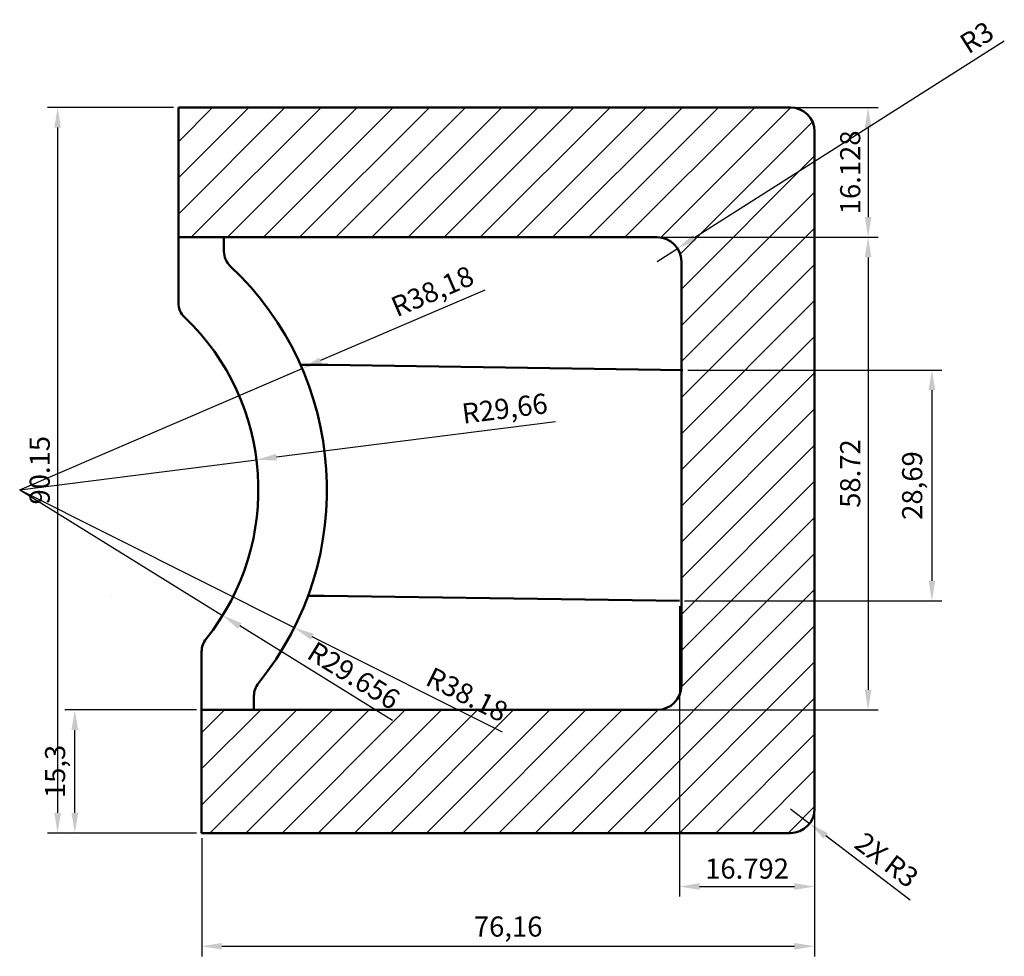
# Model space of a CAD drawing. Units: millimetres. Extents: x 1381 to 2009, y 1325 to 1613.
# Tile 6 of 6: x 1887 to 2009, y 1352 to 1468. Entities that reach past the tile are written whole.
import ezdxf

# ---------------------------------------------------------------- set-up
doc = ezdxf.new("R2010")
doc.units = ezdxf.units.MM
for name, color, linetype, lineweight in [('M-DIMS', 2, 'Continuous', 25), ('M-HATC', 8, 'Continuous', 18), ('M-OUTL', 7, 'Continuous', 50)]:
    doc.layers.add(name, color=color, linetype=linetype, lineweight=lineweight)
doc.styles.get("Standard").update_dxf_attribs({"font": 'arial.ttf'})
doc.dimstyles.new('ISO-25', dxfattribs={"dimtxt": 2.5, "dimasz": 2.5, "dimexe": 1.25, "dimexo": 0.625, "dimtad": 1, "dimtxsty": 'Standard', "dimcen": 2.5, "dimadec": 0, "dimazin": 0, "dimtfac": 1, "dimtmove": 0, "dimatfit": 3, "dimfxl": 1, "dimarcsym": 0})

# ---------------------------------------------------------------- blocks, each defined once
blk = doc.blocks.new('*D32')
at = {"layer": 'Defpoints', "color": 0, "transparency": 16777216}
for p in [(1968.55, 1439.75), (1966.02, 1438.15)]:
    blk.add_point(p, dxfattribs=at)
at = {"layer": 'M-DIMS', "color": 0, "lineweight": -2, "transparency": 16777216}
for p, q in [((2009.14, 1465.52), (1970.66, 1441.09)), ((1966.02, 1438.15), (1968.55, 1439.75))]:
    blk.add_line(p, q, dxfattribs=at)
at = {"layer": 'M-DIMS', "color": 0, "transparency": 16777216}
blk.add_solid([(1970.44, 1441.45), (1970.89, 1440.74), (1968.55, 1439.75)], dxfattribs=at)
at = {"layer": 'M-DIMS', "color": 0, "transparency": 16777216, "insert": (2005.9, 1465.71), "char_height": 2.5, "attachment_point": 5, "rotation": 32.4049}
blk.add_mtext('R3', dxfattribs=at)
blk = doc.blocks.new('*D33')
at = {"layer": 'Defpoints', "color": 0, "transparency": 16777216}
for p in [(1921.89, 1424.83), (1886.81, 1409.78)]:
    blk.add_point(p, dxfattribs=at)
at = {"layer": 'M-DIMS', "color": 0, "lineweight": -2, "transparency": 16777216}
for p, q in [((1944.6, 1434.58), (1924.19, 1425.82)), ((1886.81, 1409.78), (1921.89, 1424.83))]:
    blk.add_line(p, q, dxfattribs=at)
at = {"layer": 'M-DIMS', "color": 0, "transparency": 16777216}
blk.add_solid([(1924.02, 1426.2), (1924.35, 1425.44), (1921.89, 1424.83)], dxfattribs=at)
at = {"layer": 'M-DIMS', "color": 0, "transparency": 16777216, "insert": (1938.21, 1434.15), "char_height": 2.5, "attachment_point": 5, "rotation": 23.228}
blk.add_mtext('R38,18', dxfattribs=at)
blk = doc.blocks.new('*D34')
at = {"layer": 'Defpoints', "color": 0, "transparency": 16777216}
for p in [(1916.23, 1413.5), (1886.81, 1409.78)]:
    blk.add_point(p, dxfattribs=at)
at = {"layer": 'M-DIMS', "color": 0, "lineweight": -2, "transparency": 16777216}
for p, q in [((1953.37, 1418.21), (1918.71, 1413.82)), ((1886.81, 1409.78), (1916.23, 1413.5))]:
    blk.add_line(p, q, dxfattribs=at)
at = {"layer": 'M-DIMS', "color": 0, "transparency": 16777216}
blk.add_solid([(1918.66, 1414.23), (1918.76, 1413.41), (1916.23, 1413.5)], dxfattribs=at)
at = {"layer": 'M-DIMS', "color": 0, "transparency": 16777216, "insert": (1947.11, 1419.56), "char_height": 2.5, "attachment_point": 5, "rotation": 7.2247}
blk.add_mtext('R29,66', dxfattribs=at)
blk = doc.blocks.new('*D35')
at = {"layer": 'Defpoints', "color": 0, "transparency": 16777216}
for p in [(1969.21, 1424.65), (1968.78, 1395.96), (2000.15, 1395.96)]:
    blk.add_point(p, dxfattribs=at)
at = {"layer": 'M-DIMS', "color": 0, "lineweight": -2, "transparency": 16777216}
for p, q in [((1969.84, 1424.65), (2001.4, 1424.65)), ((2000.15, 1422.15), (2000.15, 1398.46)), ((1969.41, 1395.96), (2001.4, 1395.96))]:
    blk.add_line(p, q, dxfattribs=at)
at = {"layer": 'M-DIMS', "color": 0, "transparency": 16777216}
for points in [[(1999.73, 1422.15), (2000.56, 1422.15), (2000.15, 1424.65)], [(1999.73, 1398.46), (2000.56, 1398.46), (2000.15, 1395.96)]]:
    blk.add_solid(points, dxfattribs=at)
at = {"layer": 'M-DIMS', "color": 0, "transparency": 16777216, "insert": (1998.02, 1410.3), "char_height": 2.5, "attachment_point": 5, "rotation": 90}
blk.add_mtext('28,69', dxfattribs=at)
blk = doc.blocks.new('*D36')
at = {"layer": 'Defpoints', "color": 0, "transparency": 16777216}
for p in [(1985.57, 1370.12), (1909.42, 1367.12), (1985.57, 1353.05)]:
    blk.add_point(p, dxfattribs=at)
at = {"layer": 'M-DIMS', "color": 0, "lineweight": -2, "transparency": 16777216}
for p, q in [((1985.57, 1369.5), (1985.57, 1351.8)), ((1909.42, 1366.5), (1909.42, 1351.8)), ((1911.92, 1353.05), (1983.07, 1353.05))]:
    blk.add_line(p, q, dxfattribs=at)
at = {"layer": 'M-DIMS', "color": 0, "transparency": 16777216}
for points in [[(1911.92, 1353.47), (1911.92, 1352.64), (1909.42, 1353.05)], [(1983.07, 1353.47), (1983.07, 1352.64), (1985.57, 1353.05)]]:
    blk.add_solid(points, dxfattribs=at)
at = {"layer": 'M-DIMS', "color": 0, "transparency": 16777216, "insert": (1947.5, 1355.18), "char_height": 2.5, "attachment_point": 5}
blk.add_mtext('76,16', dxfattribs=at)
blk = doc.blocks.new('*D37')
at = {"layer": 'Defpoints', "color": 0, "transparency": 16777216}
for p in [(1893.66, 1382.42), (1909.42, 1382.42), (1909.42, 1367.12)]:
    blk.add_point(p, dxfattribs=at)
at = {"layer": 'M-DIMS', "color": 0, "lineweight": -2, "transparency": 16777216}
for p, q in [((1908.79, 1382.42), (1892.41, 1382.42)), ((1893.66, 1369.62), (1893.66, 1379.92)), ((1908.79, 1367.12), (1892.41, 1367.12))]:
    blk.add_line(p, q, dxfattribs=at)
at = {"layer": 'M-DIMS', "color": 0, "transparency": 16777216}
for points in [[(1893.24, 1379.92), (1894.08, 1379.92), (1893.66, 1382.42)], [(1893.24, 1369.62), (1894.08, 1369.62), (1893.66, 1367.12)]]:
    blk.add_solid(points, dxfattribs=at)
at = {"layer": 'M-DIMS', "color": 0, "transparency": 16777216, "insert": (1891.53, 1374.77), "char_height": 2.5, "attachment_point": 5, "rotation": 90}
blk.add_mtext('15,3', dxfattribs=at)
blk = doc.blocks.new('*D100')
at = {"layer": 'Defpoints', "color": 0, "transparency": 16777216}
for p in [(1906.52, 1457.27), (1891.52, 1367.12), (1909.42, 1367.12)]:
    blk.add_point(p, dxfattribs=at)
at = {"layer": 'M-DIMS', "color": 0, "lineweight": -2, "transparency": 16777216}
for p, q in [((1905.9, 1457.27), (1890.27, 1457.27)), ((1891.52, 1454.77), (1891.52, 1369.62)), ((1908.79, 1367.12), (1890.27, 1367.12))]:
    blk.add_line(p, q, dxfattribs=at)
at = {"layer": 'M-DIMS', "color": 0, "transparency": 16777216}
for points in [[(1891.11, 1454.77), (1891.94, 1454.77), (1891.52, 1457.27)], [(1891.11, 1369.62), (1891.94, 1369.62), (1891.52, 1367.12)]]:
    blk.add_solid(points, dxfattribs=at)
at = {"layer": 'M-DIMS', "color": 0, "transparency": 16777216, "insert": (1889.62, 1412.2), "char_height": 2.5, "attachment_point": 5, "rotation": 90}
blk.add_mtext('90.15', dxfattribs=at)
blk = doc.blocks.new('*D101')
at = {"layer": 'Defpoints', "color": 0, "transparency": 16777216}
for p in [(1906.52, 1457.27), (1906.52, 1441.15), (1992.22, 1441.15)]:
    blk.add_point(p, dxfattribs=at)
at = {"layer": 'M-DIMS', "color": 0, "lineweight": -2, "transparency": 16777216}
for p, q in [((1907.15, 1457.27), (1993.47, 1457.27)), ((1992.22, 1454.77), (1992.22, 1443.65)), ((1907.15, 1441.15), (1993.47, 1441.15))]:
    blk.add_line(p, q, dxfattribs=at)
at = {"layer": 'M-DIMS', "color": 0, "transparency": 16777216}
for points in [[(1991.81, 1454.77), (1992.64, 1454.77), (1992.22, 1457.27)], [(1991.81, 1443.65), (1992.64, 1443.65), (1992.22, 1441.15)]]:
    blk.add_solid(points, dxfattribs=at)
at = {"layer": 'M-DIMS', "color": 0, "transparency": 16777216, "insert": (1990.32, 1449.21), "char_height": 2.5, "attachment_point": 5, "rotation": 90}
blk.add_mtext('16.128', dxfattribs=at)
blk = doc.blocks.new('*D102')
at = {"layer": 'Defpoints', "color": 0, "transparency": 16777216}
for p in [(1968.78, 1395.96), (1985.57, 1370.12), (1985.57, 1360.47)]:
    blk.add_point(p, dxfattribs=at)
at = {"layer": 'M-DIMS', "color": 0, "lineweight": -2, "transparency": 16777216}
for p, q in [((1968.78, 1395.33), (1968.78, 1359.22)), ((1985.57, 1369.5), (1985.57, 1359.22)), ((1971.28, 1360.47), (1983.07, 1360.47))]:
    blk.add_line(p, q, dxfattribs=at)
at = {"layer": 'M-DIMS', "color": 0, "transparency": 16777216}
for points in [[(1971.28, 1360.89), (1971.28, 1360.06), (1968.78, 1360.47)], [(1983.07, 1360.89), (1983.07, 1360.06), (1985.57, 1360.47)]]:
    blk.add_solid(points, dxfattribs=at)
at = {"layer": 'M-DIMS', "color": 0, "transparency": 16777216, "insert": (1977.18, 1362.38), "char_height": 2.5, "attachment_point": 5}
blk.add_mtext('16.792', dxfattribs=at)
blk = doc.blocks.new('*D103')
at = {"layer": 'Defpoints', "color": 0, "transparency": 16777216}
for p in [(1966.02, 1441.15), (1966.02, 1382.42), (1992.22, 1382.42)]:
    blk.add_point(p, dxfattribs=at)
at = {"layer": 'M-DIMS', "color": 0, "lineweight": -2, "transparency": 16777216}
for p, q in [((1966.64, 1441.15), (1993.47, 1441.15)), ((1992.22, 1438.65), (1992.22, 1384.92)), ((1966.64, 1382.42), (1993.47, 1382.42))]:
    blk.add_line(p, q, dxfattribs=at)
at = {"layer": 'M-DIMS', "color": 0, "transparency": 16777216}
for points in [[(1991.81, 1438.65), (1992.64, 1438.65), (1992.22, 1441.15)], [(1991.81, 1384.92), (1992.64, 1384.92), (1992.22, 1382.42)]]:
    blk.add_solid(points, dxfattribs=at)
at = {"layer": 'M-DIMS', "color": 0, "transparency": 16777216, "insert": (1990.32, 1411.79), "char_height": 2.5, "attachment_point": 5, "rotation": 90}
blk.add_mtext('58.72', dxfattribs=at)
blk = doc.blocks.new('*D130')
at = {"layer": 'Defpoints', "color": 0, "transparency": 16777216}
for p in [(1886.81, 1409.78), (1920.92, 1392.64)]:
    blk.add_point(p, dxfattribs=at)
at = {"layer": 'M-DIMS', "color": 0, "lineweight": -2, "transparency": 16777216}
for p, q in [((1886.81, 1409.78), (1920.92, 1392.64)), ((1946.79, 1379.64), (1923.16, 1391.51))]:
    blk.add_line(p, q, dxfattribs=at)
at = {"layer": 'M-DIMS', "color": 0, "transparency": 16777216}
blk.add_solid([(1923.34, 1391.89), (1922.97, 1391.14), (1920.92, 1392.64)], dxfattribs=at)
at = {"layer": 'M-DIMS', "color": 0, "transparency": 16777216, "insert": (1942.25, 1384.05), "char_height": 2.5, "attachment_point": 5, "rotation": 333.325}
blk.add_mtext('R38.18', dxfattribs=at)
blk = doc.blocks.new('*D131')
at = {"layer": 'Defpoints', "color": 0, "transparency": 16777216}
for p in [(1886.81, 1409.78), (1912.02, 1394.17)]:
    blk.add_point(p, dxfattribs=at)
at = {"layer": 'M-DIMS', "color": 0, "lineweight": -2, "transparency": 16777216}
for p, q in [((1886.81, 1409.78), (1912.02, 1394.17)), ((1933.11, 1381.11), (1914.15, 1392.85))]:
    blk.add_line(p, q, dxfattribs=at)
at = {"layer": 'M-DIMS', "color": 0, "transparency": 16777216}
blk.add_solid([(1914.37, 1393.2), (1913.93, 1392.5), (1912.02, 1394.17)], dxfattribs=at)
at = {"layer": 'M-DIMS', "color": 0, "transparency": 16777216, "insert": (1928.15, 1386.42), "char_height": 2.5, "attachment_point": 5, "rotation": 328.2419}
blk.add_mtext('R29.656', dxfattribs=at)
blk = doc.blocks.new('*D132')
at = {"layer": 'Defpoints', "color": 0, "transparency": 16777216}
for p in [(1982.57, 1370.12), (1984.96, 1368.3)]:
    blk.add_point(p, dxfattribs=at)
at = {"layer": 'M-DIMS', "color": 0, "lineweight": -2, "transparency": 16777216}
for p, q in [((1982.57, 1370.12), (1984.96, 1368.3)), ((1997.43, 1358.78), (1986.95, 1366.79))]:
    blk.add_line(p, q, dxfattribs=at)
at = {"layer": 'M-DIMS', "color": 0, "transparency": 16777216}
blk.add_solid([(1987.2, 1367.12), (1986.69, 1366.45), (1984.96, 1368.3)], dxfattribs=at)
at = {"layer": 'M-DIMS', "color": 0, "transparency": 16777216, "insert": (1994.34, 1363.53), "char_height": 2.5, "attachment_point": 5, "rotation": 322.632}
blk.add_mtext('2X R3', dxfattribs=at)

msp = doc.modelspace()

# ---------------------------------------------------------------- hatches: boundary and pattern name
at = {"layer": 'M-HATC'}
h = msp.add_hatch(dxfattribs=at)
h.set_pattern_fill('ANSI31', color=256)
h.paths.add_polyline_path([(1985.5748, 1454.2745, 0.41421356), (1982.5748, 1457.2745), (1906.5204, 1457.2745), (1906.5204, 1441.1466), (1966.0189, 1441.1466, -0.41421356), (1969.0189, 1438.1466), (1969.0189, 1385.4245, -0.41421356), (1966.0189, 1382.4245), (1909.4177, 1382.4245), (1909.4177, 1367.1237), (1982.5748, 1367.1237, 0.41421356), (1985.5748, 1370.1237)])

# ---------------------------------------------------------------- linework, layer by layer
at = {"layer": 'M-OUTL'}
for p, q in [((1982.5748, 1457.2745), (1906.5204, 1457.2745)), ((1906.5204, 1457.2745), (1906.5204, 1441.1466)), ((1985.5748, 1370.1237), (1985.5748, 1454.2745)), ((1906.5204, 1441.1466), (1966.0189, 1441.1466)), ((1906.5204, 1441.1466), (1906.5204, 1433.0265)), ((1912.1847, 1439.399), (1912.1847, 1441.1466)), ((1969.0189, 1438.1466), (1969.0189, 1385.4245)), ((1925.0843, 1425.3057), (1921.6842, 1425.3057)), ((1925.0843, 1425.3057), (1969.2107, 1424.6476)), ((1969.0189, 1417.2453), (1969.1003, 1417.2441)), ((1898.1739, 1396.6139), (1898.1739, 1396.6139)), ((1924.6564, 1396.6139), (1922.6456, 1396.6139)), ((1924.6564, 1396.6139), (1968.7828, 1395.9558)), ((1909.4177, 1382.4245), (1909.4177, 1389.6871)), ((1915.9145, 1384.1682), (1915.9145, 1382.4245)), ((1966.0189, 1382.4245), (1909.4177, 1382.4245)), ((1909.4177, 1382.4245), (1909.4177, 1367.1237)), ((1909.4177, 1367.1237), (1982.5748, 1367.1237))]:
    msp.add_line(p, q, dxfattribs=at)
for centre, radius, start, end in [((1982.5748, 1454.2745), 3, 0, 90), ((1966.0189, 1438.1466), 3, 0, 90), ((1914.6847, 1439.399), 2.5, 180, 226.740615), ((1886.8082, 1409.7751), 38.1777, 320.986155, 46.740615), ((1909.0204, 1433.0265), 2.5, 180, 226.30943), ((1886.8082, 1409.7751), 29.6561, 321.339734, 46.30943), ((1911.9177, 1389.6871), 2.5, 141.339734, 180), ((1918.4145, 1384.1682), 2.5, 140.986155, 180), ((1966.0189, 1385.4245), 3, 270, 0), ((1982.5748, 1370.1237), 3, 270, 0)]:
    msp.add_arc(centre, radius, start, end, dxfattribs=at)

# ---------------------------------------------------------------- dimensions: what is measured, and where the dimension line sits
at = {"layer": 'M-DIMS'}
for center, mpoint, override, picture, middle in [((1966.0189, 1438.1466), (1968.5518, 1439.7543), {"dimclrd": 0, "dimclre": 0, "dimclrt": 0}, '*D32', (2006.9147, 1464.1047)), ((1886.8082, 1409.7751), (1921.8913, 1424.832), {"dimclrd": 0, "dimclre": 0, "dimclrt": 0}, '*D33', (1939.0462, 1432.1945)), ((1886.8082, 1409.7751), (1916.2288, 1413.5047), {"dimclrd": 0, "dimclre": 0, "dimclrt": 0}, '*D34', (1947.3779, 1417.4534)), ((1886.8082, 1409.7751), (1920.9225, 1392.636), {"dimdec": 2, "dimlfac": 1, "dimrnd": 0, "dimzin": 0, "dimdsep": 46, "dimlunit": 2}, '*D130', (1941.3911, 1382.3526)), ((1886.8082, 1409.7751), (1912.0241, 1394.1661), {"dimdec": 3, "dimlfac": 1, "dimrnd": 0, "dimzin": 0, "dimdsep": 46, "dimlunit": 2}, '*D131', (1927.1536, 1384.8007))]:
    dim = msp.add_radius_dim(center=center, mpoint=mpoint, dimstyle='ISO-25', override=override, dxfattribs=at)
    dim.commit()
    dim.dimension.update_dxf_attribs({"geometry": picture, "text_midpoint": middle, "dimtype": 164})
for base, p1, p2, override, picture, middle in [((1891.5239, 1367.1237), (1906.5204, 1457.2745), (1909.4177, 1367.1237), {"dimdec": 2, "dimlfac": 1, "dimrnd": 0, "dimzin": 0, "dimdsep": 46, "dimlunit": 2}, '*D100', (1889.6224, 1412.1991)), ((1992.2248, 1441.1466), (1906.5204, 1457.2745), (1906.5204, 1441.1466), {"dimdec": 3, "dimlfac": 1, "dimrnd": 0, "dimzin": 0, "dimdsep": 46, "dimlunit": 2}, '*D101', (1990.3234, 1449.2105)), ((1992.2248, 1382.4245), (1966.0189, 1441.1466), (1966.0189, 1382.4245), {"dimdec": 2, "dimlfac": 1, "dimrnd": 0, "dimzin": 0, "dimdsep": 46, "dimlunit": 2}, '*D103', (1990.3234, 1411.7856)), ((2000.1452, 1395.9558), (1969.2107, 1424.6476), (1968.7828, 1395.9558), {"dimclrd": 0, "dimclre": 0, "dimclrt": 0}, '*D35', (1998.0178, 1410.3017)), ((1893.6609, 1382.4245), (1909.4177, 1367.1237), (1909.4177, 1382.4245), {"dimclrd": 0, "dimclre": 0, "dimclrt": 0}, '*D37', (1891.5335, 1374.7741))]:
    dim = msp.add_linear_dim(base=base, p1=p1, p2=p2, angle=90, dimstyle='ISO-25', override=override, dxfattribs=at)
    dim.commit()
    dim.dimension.update_dxf_attribs({"geometry": picture, "text_midpoint": middle})
for base, p1, override, picture, middle in [((1985.5748, 1360.4737), (1968.7828, 1395.9558), {"dimdec": 3, "dimlfac": 1, "dimrnd": 0, "dimzin": 0, "dimdsep": 46, "dimlunit": 2}, '*D102', (1977.1788, 1362.3751)), ((1985.5748, 1353.0543), (1909.4177, 1367.1237), {"dimclrd": 0, "dimclre": 0, "dimclrt": 0}, '*D36', (1947.4963, 1355.1817))]:
    dim = msp.add_linear_dim(base=base, p1=p1, p2=(1985.5748, 1370.1237), dimstyle='ISO-25', override=override, dxfattribs=at)
    dim.commit()
    dim.dimension.update_dxf_attribs({"geometry": picture, "text_midpoint": middle})
dim = msp.add_radius_dim(center=(1982.5748, 1370.1237), mpoint=(1984.9591, 1368.3029), text='2X <>', dimstyle='ISO-25', override={"dimdec": 0, "dimlfac": 1, "dimrnd": 0, "dimzin": 0, "dimdsep": 46, "dimlunit": 2}, dxfattribs=at)
dim.commit()
dim.dimension.update_dxf_attribs({"geometry": '*D132', "text_midpoint": (1994.3376, 1363.5343)})

doc.saveas('drawing.dxf')
